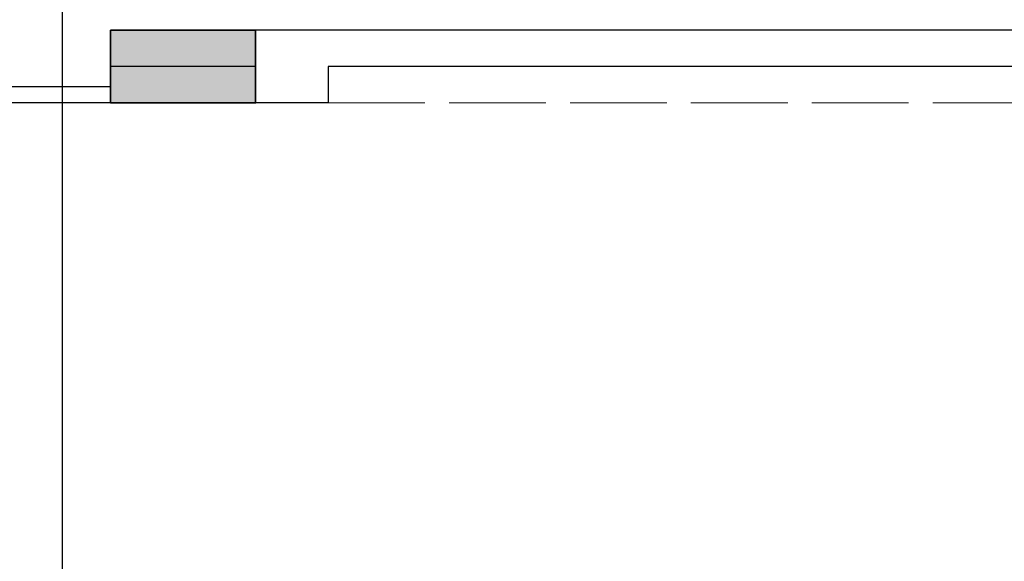
# Model space of a CAD drawing. Units: millimetres. Extents: x 595116 to 630915, y 909473 to 920225.
# Tile 10 of 134: x 629500 to 629622, y 919085 to 919152. Entities that reach past the tile are written whole.
import ezdxf

# ---------------------------------------------------------------- set-up
doc = ezdxf.new("R2010")
doc.units = ezdxf.units.MM
doc.linetypes.add('ACAD_ISO02W100', pattern=[15, 12, -3])
for name, color, linetype, lineweight in [('C-PROP', 7, 'Continuous', 25), ('C-PROP-REF', 240, 'ACAD_ISO02W100', 13), ('Column', 6, 'Continuous', 35), ('Dimension', 3, 'Continuous', 18)]:
    doc.layers.add(name, color=color, linetype=linetype, lineweight=lineweight)
doc.styles.get("Standard").update_dxf_attribs({"font": 'arial.ttf'})
doc.dimstyles.new('ISO-25', dxfattribs={"dimtxt": 9, "dimasz": 6, "dimexe": 1.25, "dimexo": 0.625, "dimtad": 1, "dimlunit": 4, "dimtxsty": 'Standard', "dimcen": 2.5, "dimadec": 0, "dimazin": 0, "dimtfac": 1, "dimtmove": 0, "dimatfit": 3, "dimfxl": 1, "dimarcsym": 0})

# ---------------------------------------------------------------- blocks, each defined once
blk = doc.blocks.new('COLUMN-RECT-18X9')
h = blk.add_hatch(color=256)
h.dxf.hatch_style = 1
h.paths.add_polyline_path([(18, 9), (0, 9), (0, 0), (18, 0)])
blk.add_lwpolyline([(0, 9), (18, 9), (18, 0), (0, 0)], close=True)
blk = doc.blocks.new('*D215')
at = {"layer": 'Defpoints', "color": 0, "transparency": 16777216}
for p in [(629316.04, 919411.83), (629505.04, 919411.83), (629505.04, 918832.38)]:
    blk.add_point(p, dxfattribs=at)
at = {"layer": 'Dimension', "color": 0, "lineweight": -2, "transparency": 16777216}
for p, q in [((629316.04, 919411.2), (629316.04, 918831.13)), ((629505.04, 919411.2), (629505.04, 918831.13)), ((629322.04, 918832.38), (629499.04, 918832.38))]:
    blk.add_line(p, q, dxfattribs=at)
at = {"layer": 'Dimension', "color": 0, "transparency": 16777216}
for points in [[(629322.04, 918833.38), (629322.04, 918831.38), (629316.04, 918832.38)], [(629499.04, 918833.38), (629499.04, 918831.38), (629505.04, 918832.38)]]:
    blk.add_solid(points, dxfattribs=at)
at = {"layer": 'Dimension', "color": 0, "transparency": 16777216, "insert": (629410.54, 918837.6), "char_height": 9, "attachment_point": 5}
blk.add_mtext('15\'-9"', dxfattribs=at)
blk = doc.blocks.new('*D216')
at = {"layer": 'Defpoints', "color": 0, "transparency": 16777216}
for p in [(629505.04, 919411.83), (629743.54, 919411.93), (629743.54, 918832.38)]:
    blk.add_point(p, dxfattribs=at)
at = {"layer": 'Dimension', "color": 0, "lineweight": -2, "transparency": 16777216}
for p, q in [((629505.04, 919411.2), (629505.04, 918831.13)), ((629743.54, 919411.3), (629743.54, 918831.13)), ((629511.04, 918832.38), (629737.54, 918832.38))]:
    blk.add_line(p, q, dxfattribs=at)
at = {"layer": 'Dimension', "color": 0, "transparency": 16777216}
for points in [[(629511.04, 918833.38), (629511.04, 918831.38), (629505.04, 918832.38)], [(629737.54, 918833.38), (629737.54, 918831.38), (629743.54, 918832.38)]]:
    blk.add_solid(points, dxfattribs=at)
at = {"layer": 'Dimension', "color": 0, "transparency": 16777216, "insert": (629624.29, 918837.66), "char_height": 9, "attachment_point": 5}
blk.add_mtext('19\'-10 1/2"', dxfattribs=at)

msp = doc.modelspace()

# ---------------------------------------------------------------- linework, layer by layer
at = {"layer": 'C-PROP'}
for p, q in [((629511.041, 919150.928), (629511.041, 919141.928)), ((629625.041, 919150.928), (629511.041, 919150.928)), ((629529.041, 919150.928), (629529.041, 919141.928)), ((629529.041, 919146.428), (629515.541, 919146.428)), ((629538.041, 919146.428), (629538.041, 919141.928)), ((629511.041, 919143.928), (629463.041, 919143.928)), ((629511.041, 919141.928), (629463.041, 919141.928))]:
    msp.add_line(p, q, dxfattribs=at)
for points in [[(629529.041, 919146.428), (629511.041, 919146.428)], [(629625.041, 919146.428), (629538.041, 919146.428)], [(629538.041, 919141.928), (629511.041, 919141.928)]]:
    msp.add_lwpolyline(points, dxfattribs=at)
at = {"layer": 'C-PROP-REF'}
for p, q in [((629529.041, 919146.428), (629511.041, 919146.428)), ((629529.041, 919141.928), (629511.041, 919141.928)), ((629625.041, 919141.928), (629538.041, 919141.928))]:
    msp.add_line(p, q, dxfattribs=at)

# ---------------------------------------------------------------- block references
at = {"layer": 'Column'}
msp.add_blockref('COLUMN-RECT-18X9', (629511.041, 919141.928), dxfattribs=at)

# ---------------------------------------------------------------- dimensions: what is measured, and where the dimension line sits
at = {"layer": 'Dimension'}
for base, p1, p2, picture, middle in [((629505.041, 918832.378), (629316.041, 919411.828), (629505.041, 919411.828), '*D215', (629410.541, 918837.598)), ((629743.541, 918832.378), (629505.041, 919411.828), (629743.541, 919411.928), '*D216', (629624.291, 918837.656))]:
    dim = msp.add_linear_dim(base=base, p1=p1, p2=p2, dimstyle='ISO-25', override={"dimdec": 1, "dimlfac": 1, "dimrnd": 0, "dimzin": 1, "dimdsep": 46, "dimlunit": 4, "dimfrac": 2}, dxfattribs=at)
    dim.commit()
    dim.dimension.update_dxf_attribs({"geometry": picture, "text_midpoint": middle})

doc.saveas('drawing.dxf')
